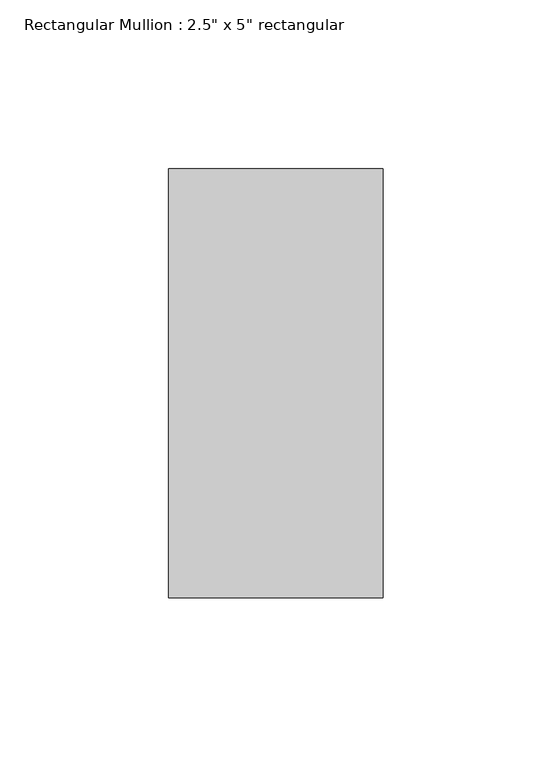
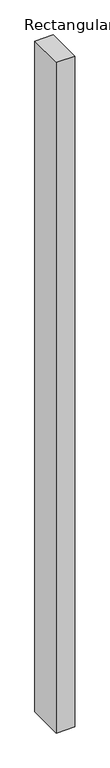
"""IFC4 building model written with IfcOpenShell, lengths in millimetres: member geometry."""

from ifc_helpers import new_model, si_unit, frame, origin, place, context, project, spatial, polyline, outline, extrude, source, transform, mapped, element, save


def member_ee409385(model_context):
    return source(origin(), model_context, "Body", "SweptSolid", [
        extrude(outline(polyline([(0.0, 63.5), (0.0, -63.5), (-63.5, -63.5), (-63.5, 63.5), (0.0, 63.5)])), frame((0.0, 0.0, -2438.4), z_axis=(0.0, 0.0, 1.0), x_axis=(1.0, 0.0, 0.0)), (0.0, 0.0, 1.0), 2438.4),
    ])


if __name__ == "__main__":
    model = new_model("IFC4")
    model_context = context("Model", 3, world=origin())
    ifc_project = project(units=[si_unit("LENGTHUNIT", "METRE", prefix="MILLI")], contexts=[model_context])
    site = spatial("IfcSite", under=ifc_project)
    building = spatial("IfcBuilding", under=site)
    placement = place(None, origin())
    member_shape = member_ee409385(model_context)
    element("IfcMember", 1, ObjectType="Rectangular Mullion : 2.5\" x 5\" rectangular", at=placement, inside=building, context=model_context, shape_type="MappedRepresentation", body=[
        mapped(member_shape, transform((0.0, 0.0, 0.0), x_axis=(1.0, 0.0, 0.0), y_axis=(0.0, 1.0, 0.0), z_axis=(0.0, 0.0, 1.0))),
    ])
    save(model, "model.ifc")

# Revit data of these elements
# Type "Rectangular Mullion : 2.5\" x 5\" rectangular"
#   built-in parameter 1007304 = 0.416667 (stored number, unit not read)
#   built-in parameter 1007301 = 0.104167 (stored number, unit not read)
#   built-in parameter 1007300 = 0.104167 (stored number, unit not read)
# Element 1 (IfcMember, "Rectangular Mullion : 2.5\" x 5\" rectangular")
#   Materials on its faces: "BLACK COLOUR"
# Materials
#   "BLACK COLOUR": class "Generic", colour RGB 120 120 120, transparency 0, Cost = 0
